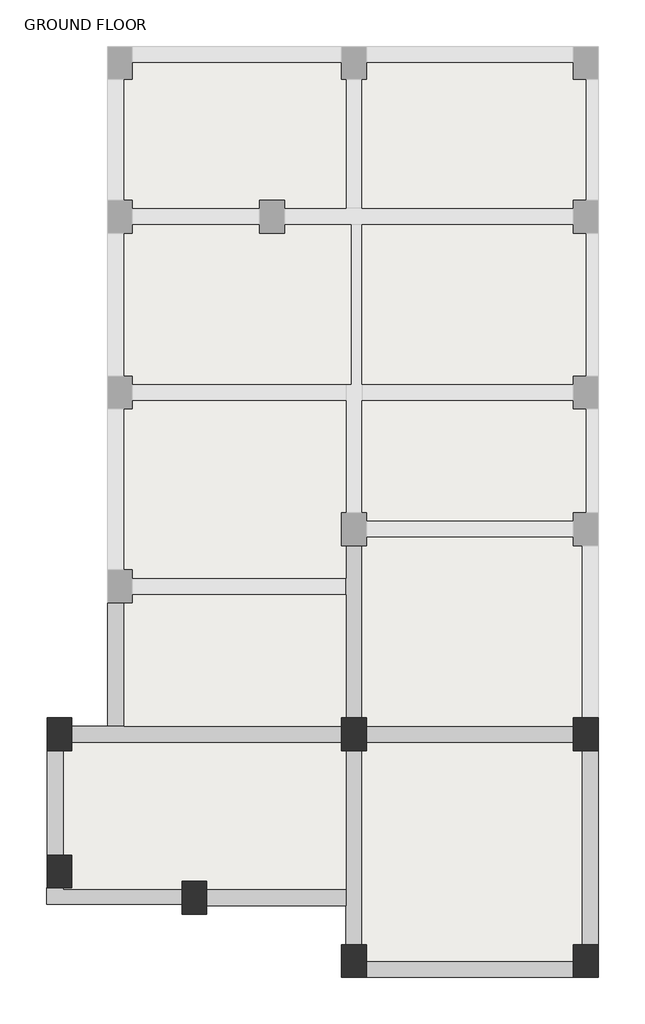
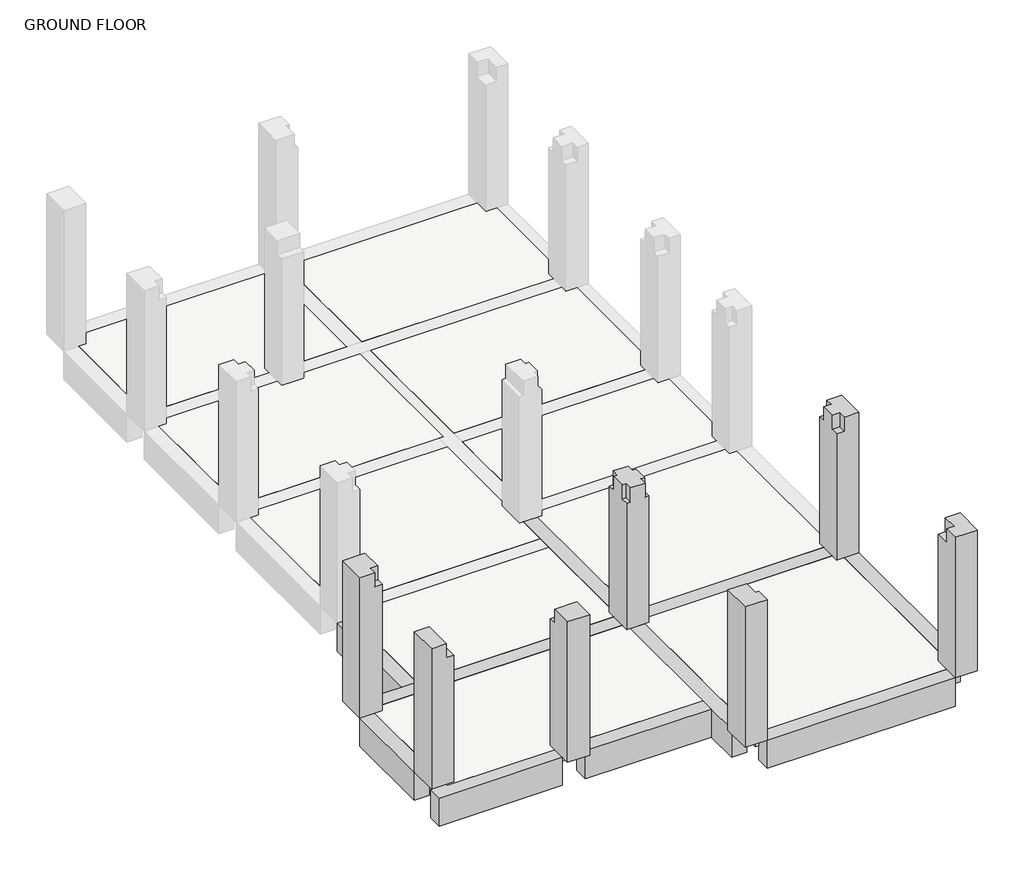
# One storey, part 1 of 2: 10 beams, 10 slabs, 7 columns.
"""IFC4 building model written with IfcOpenShell, lengths in millimetres."""

from ifc_helpers import new_model, si_unit, frame, origin, place, context, project, spatial, polyline, outline, extrude, faceted_brep, element, save

model = new_model("IFC4")

# Units and contexts
model_context = context("Model", 3, world=origin())
ifc_project = project(units=[si_unit("LENGTHUNIT", "METRE", prefix="MILLI")], contexts=[model_context])

# Site, building, storey
site = spatial("IfcSite", under=ifc_project)
building = spatial("IfcBuilding", under=site)
storey = spatial("IfcBuildingStorey", under=building, Name="GROUND FLOOR", Elevation=0.0)

# Beams
placement = place(None, origin())
element("IfcBeam", 1, ObjectType="M_Concrete-Rectangular Beam : 300 x 600mm", at=placement, inside=storey, context=model_context, shape_type="SweptSolid", body=[
    extrude(outline(polyline([(2143.5134108, -6267.3380763), (2143.5134108, -6567.3380763), (-1646.635935, -6567.3380763), (-1646.635935, -6267.3380763), (2143.5134108, -6267.3380763)])), frame((0.0, 0.0, -600.0), z_axis=(0.0, 0.0, 1.0), x_axis=(1.0, 0.0, 0.0)), (0.0, 0.0, 1.0), 600.0),
])
element("IfcBeam", 2, ObjectType="M_Concrete-Rectangular Beam : 300 x 600mm", at=placement, inside=storey, context=model_context, shape_type="SweptSolid", body=[
    extrude(outline(polyline([(2293.5134108, -2423.3693625), (2593.5134108, -2423.3693625), (2593.5134108, -5967.3380763), (2293.5134108, -5967.3380763), (2293.5134108, -2423.3693625)])), frame((0.0, 0.0, -600.0), z_axis=(0.0, 0.0, 1.0), x_axis=(1.0, 0.0, 0.0)), (0.0, 0.0, 1.0), 600.0),
])
element("IfcBeam", 3, ObjectType="M_Concrete-Rectangular Beam : 300 x 600mm", at=placement, inside=storey, context=model_context, shape_type="SweptSolid", body=[
    extrude(outline(polyline([(-1646.635935, -2273.3693625), (-1646.635935, -1973.3693625), (2143.5134108, -1973.3693625), (2143.5134108, -2273.3693625), (-1646.635935, -2273.3693625)])), frame((0.0, 0.0, -600.0), z_axis=(0.0, 0.0, 1.0), x_axis=(1.0, 0.0, 0.0)), (0.0, 0.0, 1.0), 600.0),
])
element("IfcBeam", 4, ObjectType="M_Concrete-Rectangular Beam : 300 x 600mm", at=placement, inside=storey, context=model_context, shape_type="Brep", body=[
    faceted_brep([(-1721.635935, -2423.3693625, 0.0), (-2021.635935, -2423.3693625, 0.0), (-2021.635935, -4959.2575036, 0.0), (-2021.635935, -5259.2575036, 0.0), (-2021.635935, -5967.3380763, 0.0), (-1721.635935, -5967.3380763, 0.0), (-1721.635935, -2423.3693625, -600.0), (-1721.635935, -5967.3380763, -600.0), (-2021.635935, -2423.3693625, -600.0), (-2021.635935, -5967.3380763, -600.0), (-2021.635935, -5259.2575036, -600.0), (-2021.635935, -4959.2575036, -600.0)], [[[0, 1, 2, 3, 4, 5]], [[6, 0, 5, 7]], [[8, 6, 7, 9, 10, 11]], [[1, 8, 11, 10, 9, 4, 3, 2]], [[1, 0, 6, 8]], [[4, 9, 7, 5]]]),
])
element("IfcBeam", 5, ObjectType="M_Concrete-Rectangular Beam : 300 x 600mm", at=placement, inside=storey, context=model_context, shape_type="Brep", body=[
    faceted_brep([(-1721.635935, 1328.1057379, 0.0), (-2021.635935, 1328.1057379, 0.0), (-2021.635935, 731.5941646, 0.0), (-2021.635935, 431.5941646, 0.0), (-2021.635935, -1823.3693625, 0.0), (-1721.635935, -1823.3693625, 0.0), (-1721.635935, 1328.1057379, -600.0), (-1721.635935, -1823.3693625, -600.0), (-2021.635935, 1328.1057379, -600.0), (-2021.635935, -1823.3693625, -600.0), (-2021.635935, 431.5941646, -600.0), (-2021.635935, 731.5941646, -600.0)], [[[0, 1, 2, 3, 4, 5]], [[6, 0, 5, 7]], [[8, 6, 7, 9, 10, 11]], [[1, 8, 11, 10, 9, 4, 3, 2]], [[1, 0, 6, 8]], [[4, 9, 7, 5]]]),
])
element("IfcBeam", 6, ObjectType="M_Concrete-Rectangular Beam : 300 x 600mm", at=placement, inside=storey, context=model_context, shape_type="Brep", body=[
    faceted_brep([(-4566.635935, -4959.2575036, 0.0), (-4566.635935, -5259.2575036, 0.0), (-2021.635935, -5259.2575036, 0.0), (-2021.635935, -4959.2575036, 0.0), (-4566.635935, -5259.2575036, -600.0), (-2021.635935, -5259.2575036, -600.0), (-4566.635935, -4959.2575036, -600.0), (-2021.635935, -4959.2575036, -600.0), (-2021.635935, -4959.2575036, -300.0)], [[[0, 1, 2, 3]], [[1, 4, 5, 2]], [[4, 6, 7, 5]], [[6, 0, 3, 8, 7]], [[0, 6, 4, 1]], [[3, 2, 5, 7, 8]]]),
])
element("IfcBeam", 7, ObjectType="M_Concrete-Rectangular Beam : 300 x 600mm", at=placement, inside=storey, context=model_context, shape_type="Brep", body=[
    faceted_brep([(-7032.9642664, -1973.3693625, 0.0), (-7032.9642664, -2273.3693625, 0.0), (-2096.635935, -2273.3693625, 0.0), (-2096.635935, -1973.3693625, 0.0), (-6075.9642664, -1973.3693625, 0.0), (-6375.9642664, -1973.3693625, 0.0), (-7032.9642664, -1973.3693625, -600.0), (-2096.635935, -1973.3693625, -600.0), (-6075.9642664, -1973.3693625, -600.0), (-6375.9642664, -1973.3693625, -600.0), (-7032.9642664, -2273.3693625, -600.0), (-2096.635935, -2273.3693625, -600.0)], [[[0, 1, 2, 3, 4, 5]], [[6, 0, 5, 4, 3, 7, 8, 9]], [[10, 6, 9, 8, 7, 11]], [[1, 10, 11, 2]], [[2, 11, 7, 3]], [[1, 0, 6, 10]]]),
])
element("IfcBeam", 8, ObjectType="M_Concrete-Rectangular Beam : 300 x 600mm", at=placement, inside=storey, context=model_context, shape_type="Brep", body=[
    faceted_brep([(-6075.9642664, 281.5941646, 0.0), (-6375.9642664, 281.5941646, 0.0), (-6375.9642664, -1973.3693625, 0.0), (-6075.9642664, -1973.3693625, 0.0), (-6375.9642664, 281.5941646, -600.0), (-6375.9642664, -1973.3693625, -600.0), (-6075.9642664, 281.5941646, -600.0), (-6075.9642664, -1973.3693625, -600.0), (-6075.9642664, -1973.3693625, -300.0)], [[[0, 1, 2, 3]], [[1, 4, 5, 2]], [[4, 6, 7, 5]], [[6, 0, 3, 8, 7]], [[0, 6, 4, 1]], [[3, 2, 5, 7, 8]]]),
])
element("IfcBeam", 9, ObjectType="M_Concrete-Rectangular Beam : 300 x 600mm", at=placement, inside=storey, context=model_context, shape_type="SweptSolid", body=[
    extrude(outline(polyline([(-7182.9642664, -4329.2575036), (-7482.9642664, -4329.2575036), (-7482.9642664, -2423.3693625), (-7182.9642664, -2423.3693625), (-7182.9642664, -4329.2575036)])), frame((0.0, 0.0, -600.0), z_axis=(0.0, 0.0, 1.0), x_axis=(1.0, 0.0, 0.0)), (0.0, 0.0, 1.0), 600.0),
])
element("IfcBeam", 10, ObjectType="M_Concrete-Rectangular Beam : 300 x 600mm", at=placement, inside=storey, context=model_context, shape_type="Brep", body=[
    faceted_brep([(-7496.635935, -5229.2575036, 0.0), (-7496.635935, -4929.2575036, 0.0), (-7496.635935, -4929.2575036, -600.0), (-7496.635935, -5229.2575036, -600.0), (-5016.635935, -5229.2575036, 0.0), (-5016.635935, -4959.2575036, 0.0), (-7182.9642664, -4959.2575036, 0.0), (-7182.9642664, -4929.2575036, 0.0), (-7482.9642664, -4929.2575036, 0.0), (-7182.9642664, -4929.2575036, -300.0), (-7032.9642664, -4929.2575036, -300.0), (-5016.635935, -4929.2575036, -300.0), (-5016.635935, -4929.2575036, -600.0), (-5016.635935, -5229.2575036, -600.0), (-5016.635935, -4959.2575036, -300.0), (-7182.9642664, -4959.2575036, -300.0)], [[[0, 1, 2, 3]], [[1, 0, 4, 5, 6, 7, 8]], [[2, 1, 8, 7, 9, 10, 11, 12]], [[3, 2, 12, 13]], [[0, 3, 13, 4]], [[4, 13, 12, 11, 14, 5]], [[9, 15, 14, 11, 10]], [[15, 6, 5, 14]], [[6, 15, 9, 7]]]),
])

# Columns
element("IfcColumn", 11, ObjectType="M_Concrete-Rectangular-Column : 450 x 600mm", at=placement, inside=storey, context=model_context, shape_type="SweptSolid", body=[
    extrude(outline(polyline([(0.0, -7482.9642664), (0.0, -7032.9642664), (2700.0, -7032.9642664), (2700.0, -7182.9642664), (3000.0, -7182.9642664), (3000.0, -7482.9642664), (0.0, -7482.9642664)])), frame((0.0, -4929.2575036, 0.0), z_axis=(0.0, 1.0, 0.0), x_axis=(0.0, 0.0, 1.0)), (0.0, 0.0, 1.0), 600.0),
])
element("IfcColumn", 12, ObjectType="M_Concrete-Rectangular-Column : 450 x 600mm", at=placement, inside=storey, context=model_context, shape_type="Brep", body=[
    faceted_brep([(-1646.635935, -1823.3693625, 0.0), (-1646.635935, -2423.3693625, 0.0), (-2096.635935, -2423.3693625, 0.0), (-2096.635935, -1823.3693625, 0.0), (-1646.635935, -1823.3693625, 2700.0), (-1646.635935, -1973.3693625, 2700.0), (-1646.635935, -1973.3693625, 3000.0), (-1646.635935, -2273.3693625, 3000.0), (-1646.635935, -2273.3693625, 2700.0), (-1646.635935, -2423.3693625, 2700.0), (-1721.635935, -2423.3693625, 2700.0), (-1721.635935, -2423.3693625, 3000.0), (-2021.635935, -2423.3693625, 3000.0), (-2021.635935, -2423.3693625, 2700.0), (-2096.635935, -2423.3693625, 2700.0), (-2096.635935, -2273.3693625, 2700.0), (-2096.635935, -2273.3693625, 3000.0), (-2096.635935, -1973.3693625, 3000.0), (-2096.635935, -1973.3693625, 2700.0), (-2096.635935, -1823.3693625, 2700.0), (-2021.635935, -1823.3693625, 2700.0), (-2021.635935, -1823.3693625, 3000.0), (-1721.635935, -1823.3693625, 3000.0), (-1721.635935, -1823.3693625, 2700.0), (-1721.635935, -1973.3693625, 3000.0), (-2021.635935, -1973.3693625, 3000.0), (-2021.635935, -2273.3693625, 3000.0), (-1721.635935, -2273.3693625, 3000.0), (-1721.635935, -1973.3693625, 2700.0), (-1721.635935, -2273.3693625, 2700.0), (-2021.635935, -1973.3693625, 2700.0), (-2021.635935, -2273.3693625, 2700.0)], [[[0, 1, 2, 3]], [[1, 0, 4, 5, 6, 7, 8, 9]], [[2, 1, 9, 10, 11, 12, 13, 14]], [[3, 2, 14, 15, 16, 17, 18, 19]], [[0, 3, 19, 20, 21, 22, 23, 4]], [[6, 24, 22, 21, 25, 17, 16, 26, 12, 11, 27, 7]], [[23, 28, 5, 4]], [[28, 24, 6, 5]], [[24, 28, 23, 22]], [[29, 10, 9, 8]], [[27, 29, 8, 7]], [[29, 27, 11, 10]], [[18, 30, 20, 19]], [[30, 25, 21, 20]], [[25, 30, 18, 17]], [[13, 31, 15, 14]], [[31, 26, 16, 15]], [[26, 31, 13, 12]]]),
])
element("IfcColumn", 13, ObjectType="M_Concrete-Rectangular-Column : 450 x 600mm", at=placement, inside=storey, context=model_context, shape_type="Brep", body=[
    faceted_brep([(-1646.635935, -5967.3380763, 0.0), (-1646.635935, -6567.3380763, 0.0), (-2096.635935, -6567.3380763, 0.0), (-2096.635935, -5967.3380763, 0.0), (-1646.635935, -5967.3380763, 2700.0), (-1646.635935, -6267.3380763, 2700.0), (-1646.635935, -6267.3380763, 3000.0), (-1646.635935, -6567.3380763, 3000.0), (-2096.635935, -6567.3380763, 3000.0), (-2096.635935, -5967.3380763, 3000.0), (-1721.635935, -5967.3380763, 3000.0), (-1721.635935, -5967.3380763, 2700.0), (-1721.635935, -6267.3380763, 3000.0), (-1721.635935, -6267.3380763, 2700.0)], [[[0, 1, 2, 3]], [[1, 0, 4, 5, 6, 7]], [[2, 1, 7, 8]], [[3, 2, 8, 9]], [[0, 3, 9, 10, 11, 4]], [[8, 7, 6, 12, 10, 9]], [[11, 13, 5, 4]], [[13, 12, 6, 5]], [[12, 13, 11, 10]]]),
])
element("IfcColumn", 14, ObjectType="M_Concrete-Rectangular-Column : 450 x 600mm", at=placement, inside=storey, context=model_context, shape_type="Brep", body=[
    faceted_brep([(2593.5134108, -1823.3693625, 0.0), (2593.5134108, -2423.3693625, 0.0), (2143.5134108, -2423.3693625, 0.0), (2143.5134108, -1823.3693625, 0.0), (2593.5134108, -1823.3693625, 3000.0), (2593.5134108, -2423.3693625, 3000.0), (2293.5134108, -2423.3693625, 3000.0), (2293.5134108, -2423.3693625, 2700.0), (2143.5134108, -2423.3693625, 2700.0), (2143.5134108, -2273.3693625, 2700.0), (2143.5134108, -2273.3693625, 3000.0), (2143.5134108, -1973.3693625, 3000.0), (2143.5134108, -1973.3693625, 2700.0), (2143.5134108, -1823.3693625, 2700.0), (2293.5134108, -1823.3693625, 2700.0), (2293.5134108, -1823.3693625, 3000.0), (2293.5134108, -1973.3693625, 3000.0), (2293.5134108, -2273.3693625, 3000.0), (2293.5134108, -1973.3693625, 2700.0), (2293.5134108, -2273.3693625, 2700.0)], [[[0, 1, 2, 3]], [[1, 0, 4, 5]], [[2, 1, 5, 6, 7, 8]], [[3, 2, 8, 9, 10, 11, 12, 13]], [[0, 3, 13, 14, 15, 4]], [[5, 4, 15, 16, 11, 10, 17, 6]], [[12, 18, 14, 13]], [[18, 16, 15, 14]], [[16, 18, 12, 11]], [[7, 19, 9, 8]], [[19, 17, 10, 9]], [[17, 19, 7, 6]]]),
])
element("IfcColumn", 15, ObjectType="M_Concrete-Rectangular-Column : 450 x 600mm", at=placement, inside=storey, context=model_context, shape_type="Brep", body=[
    faceted_brep([(2593.5134108, -5967.3380763, 0.0), (2593.5134108, -6567.3380763, 0.0), (2143.5134108, -6567.3380763, 0.0), (2143.5134108, -5967.3380763, 0.0), (2593.5134108, -5967.3380763, 3000.0), (2593.5134108, -6567.3380763, 3000.0), (2143.5134108, -6567.3380763, 3000.0), (2143.5134108, -6267.3380763, 3000.0), (2143.5134108, -6267.3380763, 2700.0), (2143.5134108, -5967.3380763, 2700.0), (2293.5134108, -5967.3380763, 2700.0), (2293.5134108, -5967.3380763, 3000.0), (2293.5134108, -6267.3380763, 3000.0), (2293.5134108, -6267.3380763, 2700.0)], [[[0, 1, 2, 3]], [[1, 0, 4, 5]], [[2, 1, 5, 6]], [[3, 2, 6, 7, 8, 9]], [[0, 3, 9, 10, 11, 4]], [[5, 4, 11, 12, 7, 6]], [[8, 13, 10, 9]], [[13, 12, 11, 10]], [[12, 13, 8, 7]]]),
])
element("IfcColumn", 16, ObjectType="M_Concrete-Rectangular-Column : 450 x 600mm", at=placement, inside=storey, context=model_context, shape_type="SweptSolid", body=[
    extrude(outline(polyline([(-4809.2575036, 0.0), (-5409.2575036, 0.0), (-5409.2575036, 3000.0), (-4959.2575036, 3000.0), (-4959.2575036, 2700.0), (-4809.2575036, 2700.0), (-4809.2575036, 0.0)])), frame((-5016.635935, 0.0, 0.0), z_axis=(1.0, 0.0, 0.0), x_axis=(0.0, 1.0, 0.0)), (0.0, 0.0, 1.0), 450.0),
])
element("IfcColumn", 17, ObjectType="M_Concrete-Rectangular-Column : 450 x 600mm", at=placement, inside=storey, context=model_context, shape_type="Brep", body=[
    faceted_brep([(-7032.9642664, -1823.3693625, 0.0), (-7032.9642664, -2423.3693625, 0.0), (-7482.9642664, -2423.3693625, 0.0), (-7482.9642664, -1823.3693625, 0.0), (-7032.9642664, -1823.3693625, 3000.0), (-7032.9642664, -2273.3693625, 3000.0), (-7032.9642664, -2273.3693625, 2700.0), (-7032.9642664, -2423.3693625, 2700.0), (-7182.9642664, -2423.3693625, 2700.0), (-7182.9642664, -2423.3693625, 3000.0), (-7482.9642664, -2423.3693625, 3000.0), (-7482.9642664, -1823.3693625, 3000.0), (-7182.9642664, -2273.3693625, 3000.0), (-7182.9642664, -2273.3693625, 2700.0)], [[[0, 1, 2, 3]], [[1, 0, 4, 5, 6, 7]], [[2, 1, 7, 8, 9, 10]], [[3, 2, 10, 11]], [[0, 3, 11, 4]], [[11, 10, 9, 12, 5, 4]], [[13, 8, 7, 6]], [[12, 13, 6, 5]], [[13, 12, 9, 8]]]),
])

# Slabs
element("IfcSlab", 18, ObjectType="Generic 300mm", at=placement, inside=storey, context=model_context, shape_type="SweptSolid", body=[
    extrude(outline(polyline([(-2096.635935, 10150.0657956), (-2096.635935, 9850.0657956), (-2021.635935, 9850.0657956), (-2021.635935, 7491.506653), (-3146.635935, 7491.506653), (-3146.635935, 7641.506653), (-3596.635935, 7641.506653), (-3596.635935, 7491.506653), (-5925.9642664, 7491.506653), (-5925.9642664, 7641.506653), (-6075.9642664, 7641.506653), (-6075.9642664, 9850.0657956), (-5925.9642664, 9850.0657956), (-5925.9642664, 10150.0657956), (-2096.635935, 10150.0657956)])), frame((0.0, 0.0, -300.0), z_axis=(0.0, 0.0, 1.0), x_axis=(1.0, 0.0, 0.0)), (0.0, 0.0, 1.0), 300.0),
])
element("IfcSlab", 19, ObjectType="Generic 300mm", at=placement, inside=storey, context=model_context, shape_type="Brep", body=[
    faceted_brep([(-1721.635935, 10150.0657956, -300.0), (-1646.635935, 10150.0657956, -300.0), (2143.5134108, 10150.0657956, -300.0), (2368.5134108, 10150.0657956, -300.0), (2368.5134108, 9850.0657956, -300.0), (2368.5134108, 7641.506653, -300.0), (2368.5134108, 7491.506653, -300.0), (2143.5134108, 7491.506653, -300.0), (-1721.635935, 7491.506653, -300.0), (-1721.635935, 9850.0657956, -300.0), (-1721.635935, 10150.0657956, 0.0), (-1721.635935, 9850.0657956, 0.0), (-1721.635935, 7491.506653, 0.0), (2143.5134108, 7491.506653, 0.0), (2368.5134108, 7491.506653, 0.0), (2368.5134108, 7641.506653, 0.0), (2368.5134108, 9850.0657956, 0.0), (2368.5134108, 10150.0657956, 0.0), (2143.5134108, 10150.0657956, 0.0), (-1646.635935, 10150.0657956, 0.0)], [[[0, 1, 2, 3, 4, 5, 6, 7, 8, 9]], [[10, 11, 12, 13, 14, 15, 16, 17, 18, 19]], [[3, 2, 1, 0, 10, 19, 18, 17]], [[6, 5, 4, 3, 17, 16, 15, 14]], [[8, 7, 6, 14, 13, 12]], [[0, 9, 8, 12, 11, 10]]]),
])
element("IfcSlab", 20, ObjectType="Generic 300mm", at=placement, inside=storey, context=model_context, shape_type="Brep", body=[
    faceted_brep([(-1721.635935, 7191.506653, -300.0), (2143.5134108, 7191.506653, -300.0), (2368.5134108, 7191.506653, -300.0), (2368.5134108, 7041.506653, -300.0), (2368.5134108, 4424.5351605, -300.0), (2368.5134108, 4274.5351605, -300.0), (2143.5134108, 4274.5351605, -300.0), (-1721.635935, 4274.5351605, -300.0), (-1721.635935, 7191.506653, 0.0), (-1721.635935, 4274.5351605, 0.0), (2143.5134108, 4274.5351605, 0.0), (2368.5134108, 4274.5351605, 0.0), (2368.5134108, 4424.5351605, 0.0), (2368.5134108, 7041.506653, 0.0), (2368.5134108, 7191.506653, 0.0), (2143.5134108, 7191.506653, 0.0)], [[[0, 1, 2, 3, 4, 5, 6, 7]], [[8, 9, 10, 11, 12, 13, 14, 15]], [[2, 1, 0, 8, 15, 14]], [[5, 4, 3, 2, 14, 13, 12, 11]], [[7, 6, 5, 11, 10, 9]], [[0, 7, 9, 8]]]),
])
element("IfcSlab", 21, ObjectType="Generic 300mm", at=placement, inside=storey, context=model_context, shape_type="Brep", body=[
    faceted_brep([(-6075.9642664, 7191.506653, -300.0), (-5925.9642664, 7191.506653, -300.0), (-3596.635935, 7191.506653, -300.0), (-3146.635935, 7191.506653, -300.0), (-2021.635935, 7191.506653, -300.0), (-1928.7254278, 7191.506653, -300.0), (-1928.7254278, 4274.5351605, -300.0), (-2021.635935, 4274.5351605, -300.0), (-5925.9642664, 4274.5351605, -300.0), (-6075.9642664, 4274.5351605, -300.0), (-6075.9642664, 4424.5351605, -300.0), (-6075.9642664, 7041.506653, -300.0), (-6075.9642664, 7191.506653, 0.0), (-6075.9642664, 7041.506653, 0.0), (-6075.9642664, 4424.5351605, 0.0), (-6075.9642664, 4274.5351605, 0.0), (-5925.9642664, 4274.5351605, 0.0), (-2021.635935, 4274.5351605, 0.0), (-1928.7254278, 4274.5351605, 0.0), (-1928.7254278, 7191.506653, 0.0), (-3146.635935, 7191.506653, 0.0), (-3596.635935, 7191.506653, 0.0), (-5925.9642664, 7191.506653, 0.0)], [[[0, 1, 2, 3, 4, 5, 6, 7, 8, 9, 10, 11]], [[12, 13, 14, 15, 16, 17, 18, 19, 20, 21, 22]], [[5, 4, 3, 2, 1, 0, 12, 22, 21, 20, 19]], [[6, 5, 19, 18]], [[9, 8, 7, 6, 18, 17, 16, 15]], [[0, 11, 10, 9, 15, 14, 13, 12]]]),
])
element("IfcSlab", 22, ObjectType="Generic 300mm", at=placement, inside=storey, context=model_context, shape_type="Brep", body=[
    faceted_brep([(-1721.635935, 3974.5351605, -300.0), (2143.5134108, 3974.5351605, -300.0), (2368.5134108, 3974.5351605, -300.0), (2368.5134108, 3824.5351605, -300.0), (2368.5134108, 1928.1057379, -300.0), (2368.5134108, 1778.1057379, -300.0), (2143.5134108, 1778.1057379, -300.0), (-1646.635935, 1778.1057379, -300.0), (-1721.635935, 1778.1057379, -300.0), (-1721.635935, 1928.1057379, -300.0), (-1721.635935, 3974.5351605, 0.0), (-1721.635935, 1928.1057379, 0.0), (-1721.635935, 1778.1057379, 0.0), (-1646.635935, 1778.1057379, 0.0), (2143.5134108, 1778.1057379, 0.0), (2368.5134108, 1778.1057379, 0.0), (2368.5134108, 1928.1057379, 0.0), (2368.5134108, 3824.5351605, 0.0), (2368.5134108, 3974.5351605, 0.0), (2143.5134108, 3974.5351605, 0.0)], [[[0, 1, 2, 3, 4, 5, 6, 7, 8, 9]], [[10, 11, 12, 13, 14, 15, 16, 17, 18, 19]], [[2, 1, 0, 10, 19, 18]], [[5, 4, 3, 2, 18, 17, 16, 15]], [[8, 7, 6, 5, 15, 14, 13, 12]], [[0, 9, 8, 12, 11, 10]]]),
])
element("IfcSlab", 23, ObjectType="Generic 300mm", at=placement, inside=storey, context=model_context, shape_type="Brep", body=[
    faceted_brep([(-1721.635935, 1478.1057379, -300.0), (-1646.635935, 1478.1057379, -300.0), (2143.5134108, 1478.1057379, -300.0), (2293.5134108, 1478.1057379, -300.0), (2293.5134108, 1328.1057379, -300.0), (2293.5134108, -1823.3693625, -300.0), (2293.5134108, -1973.3693625, -300.0), (2143.5134108, -1973.3693625, -300.0), (-1646.635935, -1973.3693625, -300.0), (-1721.635935, -1973.3693625, -300.0), (-1721.635935, -1823.3693625, -300.0), (-1721.635935, 1328.1057379, -300.0), (-1721.635935, 1478.1057379, 0.0), (-1721.635935, 1328.1057379, 0.0), (-1721.635935, -1823.3693625, 0.0), (-1721.635935, -1973.3693625, 0.0), (-1646.635935, -1973.3693625, 0.0), (2143.5134108, -1973.3693625, 0.0), (2293.5134108, -1973.3693625, 0.0), (2293.5134108, -1823.3693625, 0.0), (2293.5134108, 1328.1057379, 0.0), (2293.5134108, 1478.1057379, 0.0), (2143.5134108, 1478.1057379, 0.0), (-1646.635935, 1478.1057379, 0.0)], [[[0, 1, 2, 3, 4, 5, 6, 7, 8, 9, 10, 11]], [[12, 13, 14, 15, 16, 17, 18, 19, 20, 21, 22, 23]], [[3, 2, 1, 0, 12, 23, 22, 21]], [[6, 5, 4, 3, 21, 20, 19, 18]], [[9, 8, 7, 6, 18, 17, 16, 15]], [[0, 11, 10, 9, 15, 14, 13, 12]]]),
])
element("IfcSlab", 24, ObjectType="Generic 300mm", at=placement, inside=storey, context=model_context, shape_type="Brep", body=[
    faceted_brep([(-1721.635935, -2273.3693625, -300.0), (-1646.635935, -2273.3693625, -300.0), (2143.5134108, -2273.3693625, -300.0), (2293.5134108, -2273.3693625, -300.0), (2293.5134108, -2423.3693625, -300.0), (2293.5134108, -5967.3380763, -300.0), (2293.5134108, -6267.3380763, -300.0), (2143.5134108, -6267.3380763, -300.0), (-1646.635935, -6267.3380763, -300.0), (-1721.635935, -6267.3380763, -300.0), (-1721.635935, -5967.3380763, -300.0), (-1721.635935, -2423.3693625, -300.0), (-1721.635935, -2273.3693625, 0.0), (-1721.635935, -2423.3693625, 0.0), (-1721.635935, -5967.3380763, 0.0), (-1721.635935, -6267.3380763, 0.0), (-1646.635935, -6267.3380763, 0.0), (2143.5134108, -6267.3380763, 0.0), (2293.5134108, -6267.3380763, 0.0), (2293.5134108, -5967.3380763, 0.0), (2293.5134108, -2423.3693625, 0.0), (2293.5134108, -2273.3693625, 0.0), (2143.5134108, -2273.3693625, 0.0), (-1646.635935, -2273.3693625, 0.0)], [[[0, 1, 2, 3, 4, 5, 6, 7, 8, 9, 10, 11]], [[12, 13, 14, 15, 16, 17, 18, 19, 20, 21, 22, 23]], [[3, 2, 1, 0, 12, 23, 22, 21]], [[6, 5, 4, 3, 21, 20, 19, 18]], [[9, 8, 7, 6, 18, 17, 16, 15]], [[0, 11, 10, 9, 15, 14, 13, 12]]]),
])
element("IfcSlab", 25, ObjectType="Generic 300mm", at=placement, inside=storey, context=model_context, shape_type="Brep", body=[
    faceted_brep([(-6075.9642664, 3974.5351605, -300.0), (-5925.9642664, 3974.5351605, -300.0), (-2021.635935, 3974.5351605, -300.0), (-2021.635935, 1928.1057379, -300.0), (-2021.635935, 1328.1057379, -300.0), (-2021.635935, 731.5941646, -300.0), (-5925.9642664, 731.5941646, -300.0), (-6075.9642664, 731.5941646, -300.0), (-6075.9642664, 881.5941646, -300.0), (-6075.9642664, 3824.5351605, -300.0), (-6075.9642664, 3974.5351605, 0.0), (-6075.9642664, 3824.5351605, 0.0), (-6075.9642664, 881.5941646, 0.0), (-6075.9642664, 731.5941646, 0.0), (-5925.9642664, 731.5941646, 0.0), (-2021.635935, 731.5941646, 0.0), (-2021.635935, 1328.1057379, 0.0), (-2021.635935, 1928.1057379, 0.0), (-2021.635935, 3974.5351605, 0.0), (-5925.9642664, 3974.5351605, 0.0)], [[[0, 1, 2, 3, 4, 5, 6, 7, 8, 9]], [[10, 11, 12, 13, 14, 15, 16, 17, 18, 19]], [[2, 1, 0, 10, 19, 18]], [[5, 4, 3, 2, 18, 17, 16, 15]], [[7, 6, 5, 15, 14, 13]], [[0, 9, 8, 7, 13, 12, 11, 10]]]),
])
element("IfcSlab", 26, ObjectType="Generic 300mm", at=placement, inside=storey, context=model_context, shape_type="Brep", body=[
    faceted_brep([(-6075.9642664, 431.5941646, -300.0), (-5925.9642664, 431.5941646, -300.0), (-2021.635935, 431.5941646, -300.0), (-2021.635935, -1823.3693625, -300.0), (-2021.635935, -1973.3693625, -300.0), (-2096.635935, -1973.3693625, -300.0), (-6075.9642664, -1973.3693625, -300.0), (-6075.9642664, 281.5941646, -300.0), (-6075.9642664, 431.5941646, 0.0), (-6075.9642664, 281.5941646, 0.0), (-6075.9642664, -1973.3693625, 0.0), (-2096.635935, -1973.3693625, 0.0), (-2021.635935, -1973.3693625, 0.0), (-2021.635935, -1823.3693625, 0.0), (-2021.635935, 431.5941646, 0.0), (-5925.9642664, 431.5941646, 0.0)], [[[0, 1, 2, 3, 4, 5, 6, 7]], [[8, 9, 10, 11, 12, 13, 14, 15]], [[2, 1, 0, 8, 15, 14]], [[4, 3, 2, 14, 13, 12]], [[6, 5, 4, 12, 11, 10]], [[0, 7, 6, 10, 9, 8]]]),
])
element("IfcSlab", 27, ObjectType="Generic 300mm", at=placement, inside=storey, context=model_context, shape_type="Brep", body=[
    faceted_brep([(-7182.9642664, -2273.3693625, -300.0), (-7032.9642664, -2273.3693625, -300.0), (-2096.635935, -2273.3693625, -300.0), (-2021.635935, -2273.3693625, -300.0), (-2021.635935, -2423.3693625, -300.0), (-2021.635935, -4959.2575036, -300.0), (-4566.635935, -4959.2575036, -300.0), (-5016.635935, -4959.2575036, -300.0), (-7182.9642664, -4959.2575036, -300.0), (-7182.9642664, -4929.2575036, -300.0), (-7182.9642664, -4329.2575036, -300.0), (-7182.9642664, -2423.3693625, -300.0), (-7182.9642664, -2273.3693625, 0.0), (-7182.9642664, -2423.3693625, 0.0), (-7182.9642664, -4329.2575036, 0.0), (-7182.9642664, -4929.2575036, 0.0), (-7182.9642664, -4959.2575036, 0.0), (-5016.635935, -4959.2575036, 0.0), (-4566.635935, -4959.2575036, 0.0), (-2021.635935, -4959.2575036, 0.0), (-2021.635935, -2423.3693625, 0.0), (-2021.635935, -2273.3693625, 0.0), (-2096.635935, -2273.3693625, 0.0), (-7032.9642664, -2273.3693625, 0.0)], [[[0, 1, 2, 3, 4, 5, 6, 7, 8, 9, 10, 11]], [[12, 13, 14, 15, 16, 17, 18, 19, 20, 21, 22, 23]], [[3, 2, 1, 0, 12, 23, 22, 21]], [[5, 4, 3, 21, 20, 19]], [[8, 7, 6, 5, 19, 18, 17, 16]], [[0, 11, 10, 9, 8, 16, 15, 14, 13, 12]]]),
])

save(model, "model.ifc")

# Revit data of these elements
# Type "M_Concrete-Rectangular Beam : 300 x 600mm"
#   Length [instance default] = 1524 mm
#   b = 300 mm
#   h = 600 mm
#   Structural Material [instance default] = Concrete, Cast-in-Place gray
#   Assembly Code = ""
# Type "M_Concrete-Rectangular-Column : 450 x 600mm"
#   b = 450 mm
#   h = 600 mm
#   Structural Material [instance default] = Concrete, Cast-in-Place gray
# Type "Generic 300mm"
#   Function = 0
#   Layers, outside or top first: 300 mm no material (function 1)
# Elements 1, 2, 3, 4, 5, 6, 7, 8, 9, 10 (IfcBeam, "M_Concrete-Rectangular Beam : 300 x 600mm")
#   Structural Material = Concrete, Cast-in-Place gray
#   Phase Created = New Construction
#   Materials on its faces: "Concrete, Cast-in-Place gray"
# Elements 11, 12, 13, 14, 15, 16, 17 (IfcColumn, "M_Concrete-Rectangular-Column : 450 x 600mm")
#   Structural Material = Concrete, Cast-in-Place gray
#   Phase Created = New Construction
#   Materials on its faces: "Concrete, Cast-in-Place gray"
# Element 18 (IfcSlab, "Generic 300mm")
#   Height Offset From Level = 0 mm
#   built-in parameter 1001954 = 1
#   Phase Created = New Construction
#   Materials on its faces: "Default Floor"
# Elements 19, 20, 21, 22, 23, 24, 25, 26, 27 (IfcSlab, "Generic 300mm")
#   built-in parameter 1001955 = 3.14159 (stored number, unit not read)
#   Height Offset From Level = 0 mm
#   built-in parameter 1001954 = 1
#   Phase Created = New Construction
#   Materials on its faces: "Default Floor"
# Materials
#   "Concrete, Cast-in-Place gray": class "Concrete", colour RGB 192 192 192, transparency 0, Description = "Cast-in-place concrete", Cost = 0
#   "Default Floor": colour RGB 127 127 127, transparency 0, Cost = 0
